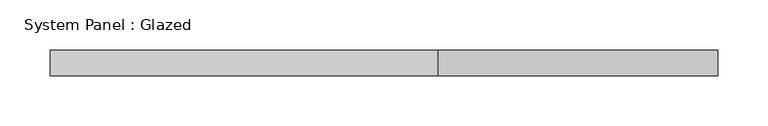
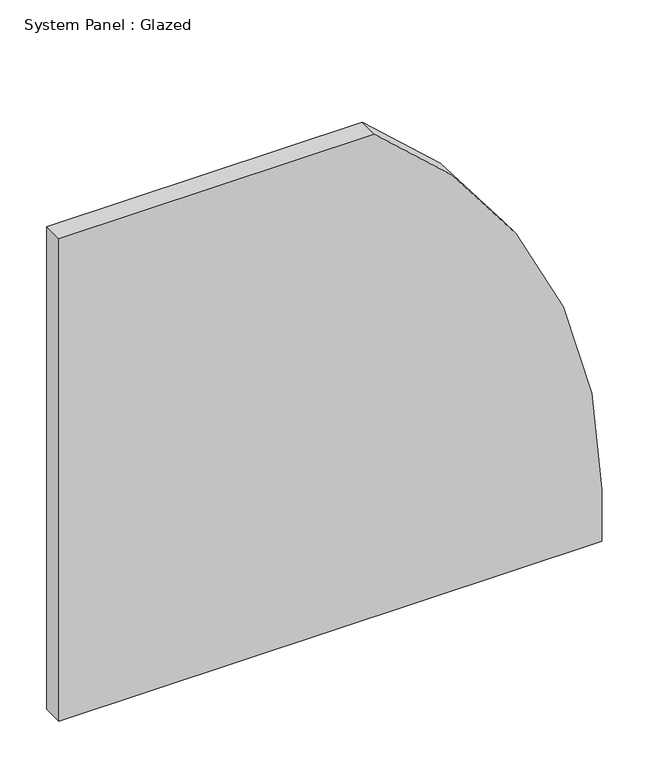
"""IFC4 building model written with IfcOpenShell, lengths in millimetres: plate geometry, System Panel : Glazed."""

from ifc_helpers import new_model, si_unit, point, frame, frame_2d, origin, place, context, project, spatial, polyline, circle_curve, trimmed, segment, composite_curve, outline, extrude, source, transform, mapped, element, save


def system_panel_glazed_dbe48e5a(model_context):
    return source(origin(), model_context, "Body", "SweptSolid", [
        extrude(outline(composite_curve([segment(polyline([(0.0, -333.375), (0.0, 333.375), (67.7333333, 333.375)]), True, "CONTINUOUS"), segment(trimmed(circle_curve(frame_2d((67.7333333, -365.125)), 698.5), [point((67.7333333, 333.375))], [point((626.5333333, 53.975))], False, "CARTESIAN"), True, "CONTINUOUS"), segment(polyline([(626.5333333, 53.975), (626.5333333, -333.375), (0.0, -333.375)]), True, "CONTINUOUS")], self_intersect=False)), frame((0.0, 19.05, 0.0), z_axis=(0.0, 1.0, 0.0), x_axis=(0.0, 0.0, 1.0)), (0.0, 0.0, 1.0), 25.4),
    ])


if __name__ == "__main__":
    model = new_model("IFC4")
    model_context = context("Model", 3, world=origin())
    ifc_project = project(units=[si_unit("LENGTHUNIT", "METRE", prefix="MILLI")], contexts=[model_context])
    site = spatial("IfcSite", under=ifc_project)
    building = spatial("IfcBuilding", under=site)
    placement = place(None, origin())
    system_panel_glazed_shape = system_panel_glazed_dbe48e5a(model_context)
    element("IfcPlate", 1, ObjectType="System Panel : Glazed", at=placement, inside=building, context=model_context, shape_type="MappedRepresentation", body=[
        mapped(system_panel_glazed_shape, transform((0.0, 0.0, 0.0), x_axis=(1.0, 0.0, 0.0), y_axis=(0.0, 1.0, 0.0), z_axis=(0.0, 0.0, 1.0))),
    ])
    save(model, "model.ifc")

# Revit data of these elements
# Type "System Panel : Glazed"
#   Construction Type Id = "GSP4R"
#   Analytic Construction = "1/8 in Pilkington single glazing"
#   Visual Light Transmittance = 0.9
#   Solar Heat Gain Coefficient = 0.86
#   Heat Transfer Coefficient (U) = 1.18115 BTU/(h·ft²·°F)
#   Define Thermal Properties by = 1
# Element 1 (IfcPlate, "System Panel : Glazed")
#   Materials on its faces: "Glass"
# Materials
#   "Glass": class "Glass", colour RGB 0 128 192, transparency 0.75, Description = "Soda Lime Glass", Cost = 0
